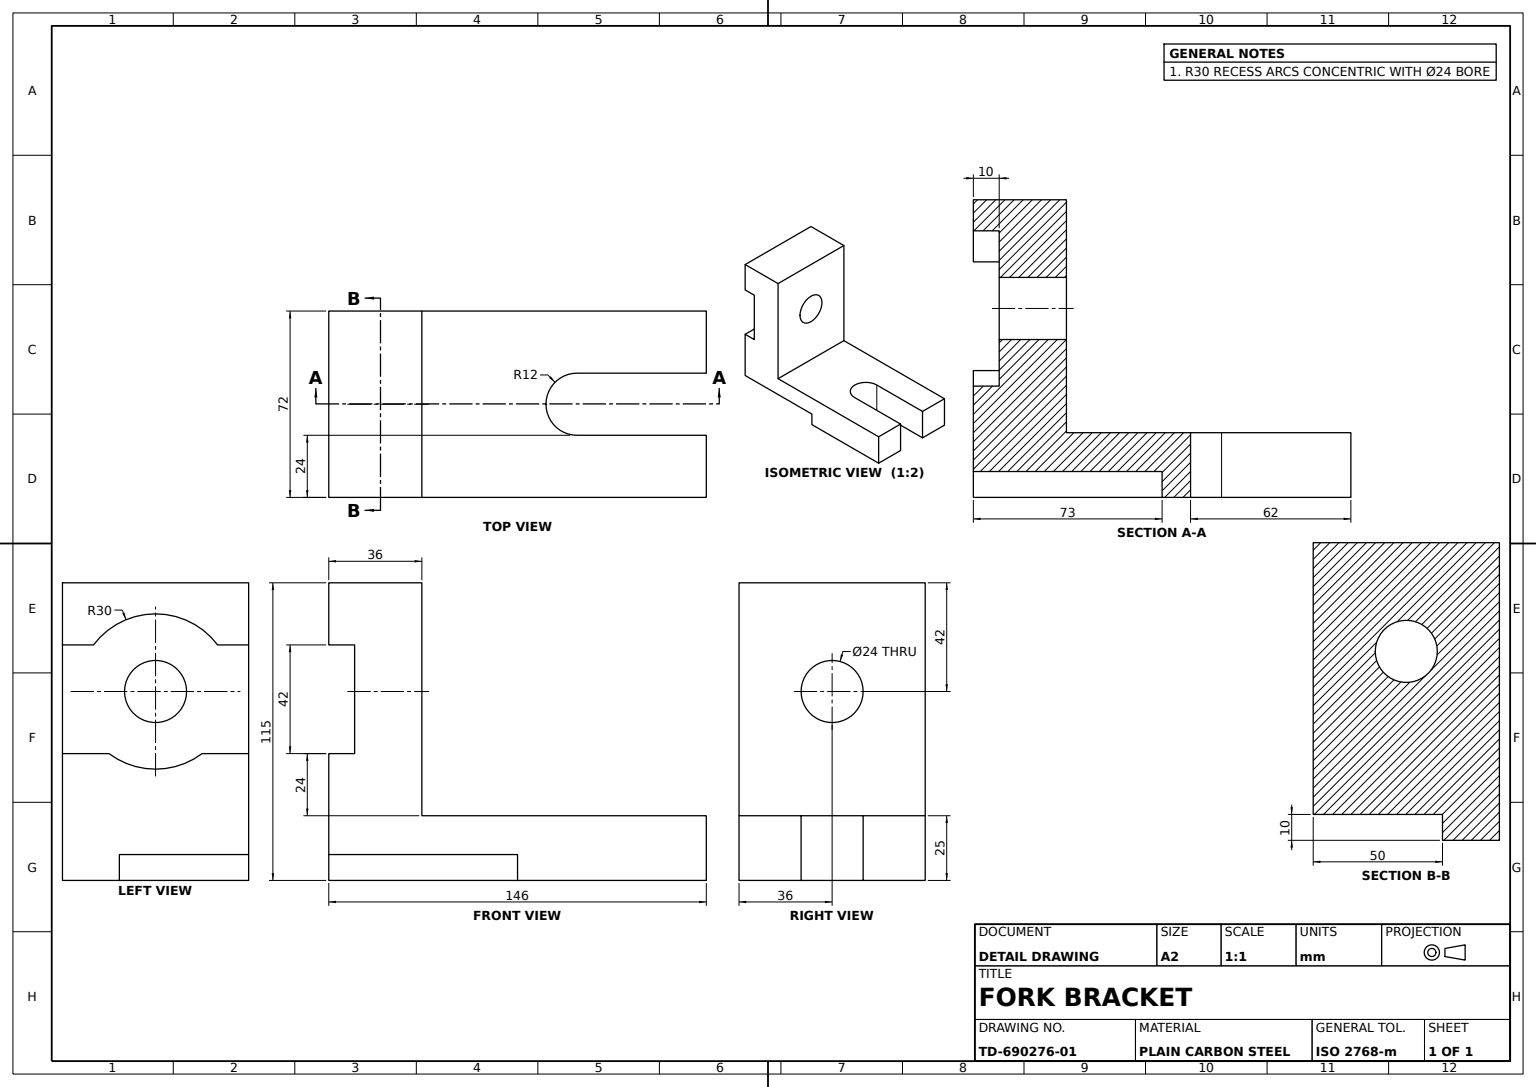
SolidWorks part; units mm, degrees
material "Plain Carbon Steel"
ref_plane "Front Plane" through (0, 0, 0) normal (0, 0, 1) x (1, 0, 0)
ref_plane "Top Plane" through (0, 0, 0) normal (0, 1, 0) x (1, 0, 0)
ref_plane "Right Plane" through (0, 0, 0) normal (1, 0, 0) x (0, 0, -1)
sketch "Upright Block Profile" plane through (0, 0, 0) normal (0, 0, 1) x (1, 0, 0)
  line L0 (-196.6364, 0) -> (196.6364, 0) construction
  line L2 (0, 0) -> (72, 0)
  line L3 (0, 0) -> (0, 90)
  line L4 (0, 90) -> (72, 90)
  line L5 (72, 0) -> (72, 90)
  point P4 (0, 0)
  dimension "D1" = 90
  dimension "D2" = 72
extrude "Upright Block" add sketch "Upright Block Profile" against normal blind 36
sketch "Side Recess Sketch" plane through (0, 0, 0) normal (0, 0, 1) x (1, 0, 0)
  line L0 (0, 0) -> (72, 0) construction
  line L1 (0, 66) -> (12, 66)
  line L2 (0, 90) -> (0, 0) construction
  line L3 (72, 0) -> (72, 90) construction
  line L4 (72, 90) -> (0, 90) construction
  line L5 (0, 24) -> (18, 24)
  line L6 (60, 66) -> (72, 66)
  line L7 (54, 24) -> (72, 24)
  line L8 (0, 66) -> (0, 24)
  line L9 (72, 24) -> (72, 66)
  arc A0 (18, 24) -> (54, 24) centre (36, 48) ccw
  arc A1 (60, 66) -> (12, 66) centre (36, 48) ccw
  dimension "D1" = 60
  dimension "D2" = 48
  dimension "D3" = 24
  dimension "D4" = 24
extrude "Side Recess 10 Deep" cut sketch "Side Recess Sketch" against normal blind 10
sketch "Bore Sketch" plane through (0, 0, -10) normal (0, 0, 1) x (1, 0, 0)
  circle A0 centre (36, 48) radius 12
  dimension "D1" = 24
extrude "Bore Ø24" cut sketch "Bore Sketch" against normal blind 42 contours A0
sketch "Base Arm Sketch" plane through (72, 0, 0) normal (1, 0, 0) x (0, 0, -1)
  line L0 (0, 0) -> (0, -25)
  line L1 (0, -25) -> (146, -25)
  line L2 (146, -25) -> (146, 0)
  line L3 (146, 0) -> (0, 0)
  dimension "D1" = 146
  dimension "D2" = 25
extrude "Base Arm 146x25" add sketch "Base Arm Sketch" against normal up to surface (72 mm away) up to face at (0, 45, -11.5)
sketch "Arm Slot Sketch" plane through (0, 0, 0) normal (0, 1, 0) x (1, 0, 0)
  line L0 (0, 146) -> (0, 36) construction
  line L1 (0, 146) -> (72, 146) construction
  line L2 (24, 146) -> (24, 96)
  line L3 (48, 96) -> (48, 146)
  line L5 (24, 146) -> (48, 146)
  arc A0 (24, 96) -> (48, 96) centre (36, 96) ccw
  point P0 (36, 84)
  dimension "D3" = 36
  dimension "D2" = 12
  dimension "D1" = 62
extrude "Arm Slot" cut sketch "Arm Slot Sketch" against normal blind 42
sketch "Relief Groove Sketch" plane through (0, 0, 0) normal (0, 0, 1) x (1, 0, 0)
  line L1 (72, -25) -> (22, -25)
  line L2 (72, -25) -> (72, -15)
  line L3 (72, -15) -> (22, -15)
  line L4 (22, -25) -> (22, -15)
  dimension "D1" = 10
  dimension "D2" = 50
extrude "Underside Relief Groove 10x50" cut sketch "Relief Groove Sketch" against normal blind 73
